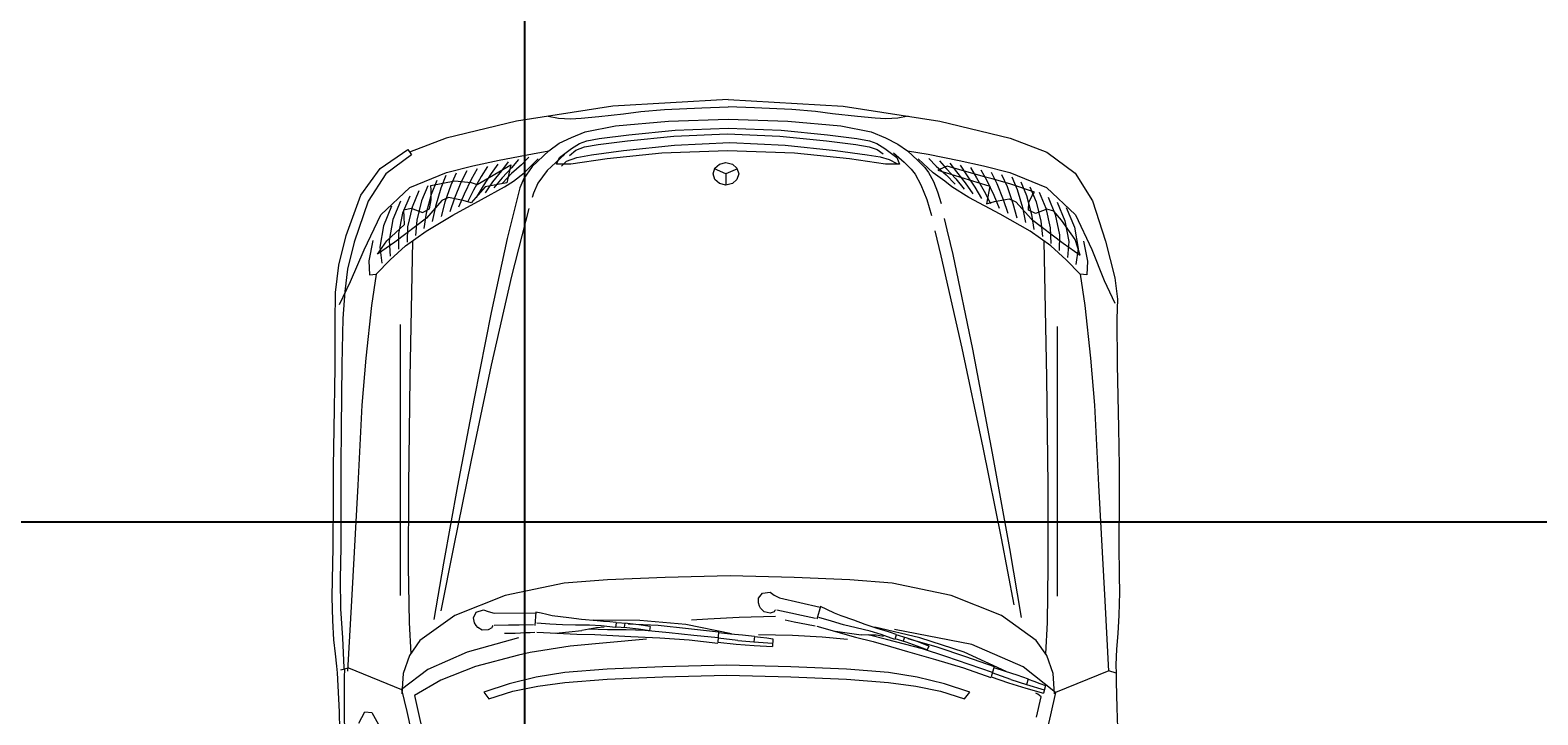
# Model space of a CAD drawing. Units: inches. Extents: x -4347 to -3836, y 955 to 1521.
# Tile 5 of 11: x -4144 to -4072, y 1088 to 1120. Entities that reach past the tile are written whole.
import ezdxf

# ---------------------------------------------------------------- set-up
doc = ezdxf.new("R2010")
doc.units = ezdxf.units.IN
doc.header["$MEASUREMENT"] = 0
doc.layers.add('A-ANNO-DIMS', color=2, linetype='Continuous', lineweight=18)
doc.layers.add('A-SITE-VEHC', color=8, linetype='Continuous', lineweight=13)
doc.styles.get("Standard").update_dxf_attribs({"font": 'arial.ttf'})
doc.dimstyles.get("Standard").update_dxf_attribs({"dimtxt": 0.18, "dimasz": 0.18, "dimexe": 0.18, "dimexo": 0.0625, "dimgap": 0.09, "dimtad": 0, "dimtih": 1, "dimtoh": 1, "dimdec": 0, "dimzin": 0, "dimdsep": 46, "dimlunit": 3, "dimtxsty": 'Standard', "dimcen": 0.09, "dimadec": 0, "dimazin": 0, "dimtfac": 1, "dimtdec": 0, "dimtofl": 0, "dimtmove": 0, "dimatfit": 3, "dimfxl": 1, "dimtolj": 1, "dimtzin": 0, "dimarcsym": 0})

# ---------------------------------------------------------------- blocks, each defined once
blk = doc.blocks.new('*D47')
at = {"layer": 'A-ANNO-DIMS', "color": 0, "lineweight": -2, "transparency": 16777216}
for p, q in [((-4120.58, 1288.726), (-4120.58, 966.959)), ((-3940.58, 1288.726), (-3940.58, 966.959)), ((-4120.4, 967.139), (-4030.97, 967.139)), ((-3940.76, 967.139), (-4030.189, 967.139))]:
    blk.add_line(p, q, dxfattribs=at)
at = {"layer": 'A-ANNO-DIMS', "color": 0, "transparency": 16777216}
for points in [[(-4120.4, 967.169), (-4120.4, 967.109), (-4120.58, 967.139)], [(-3940.76, 967.169), (-3940.76, 967.109), (-3940.58, 967.139)]]:
    blk.add_solid(points, dxfattribs=at)
at = {"layer": 'Defpoints', "color": 0, "transparency": 16777216}
for p in [(-4120.58, 1288.789), (-3940.58, 1288.789), (-3940.58, 967.139)]:
    blk.add_point(p, dxfattribs=at)
at = {"layer": 'A-ANNO-DIMS', "color": 0, "transparency": 16777216, "insert": (-4030.58, 967.139), "char_height": 0.18, "attachment_point": 5}
blk.add_mtext('\\A1;15\'-0"', dxfattribs=at)
blk = doc.blocks.new('*D54')
at = {"layer": 'A-ANNO-DIMS', "color": 0, "lineweight": -2, "transparency": 16777216}
for p, q in [((-3997.757, 1126.789), (-4346.41, 1126.789)), ((-4346.23, 1126.609), (-4346.23, 1111.971)), ((-4346.23, 1096.969), (-4346.23, 1111.607)), ((-3997.757, 1096.789), (-4346.41, 1096.789))]:
    blk.add_line(p, q, dxfattribs=at)
at = {"layer": 'A-ANNO-DIMS', "color": 0, "transparency": 16777216}
for points in [[(-4346.26, 1126.609), (-4346.2, 1126.609), (-4346.23, 1126.789)], [(-4346.26, 1096.969), (-4346.2, 1096.969), (-4346.23, 1096.789)]]:
    blk.add_solid(points, dxfattribs=at)
at = {"layer": 'Defpoints', "color": 0, "transparency": 16777216}
for p in [(-4346.23, 1126.789), (-3997.694, 1126.789), (-3997.694, 1096.789)]:
    blk.add_point(p, dxfattribs=at)
at = {"layer": 'A-ANNO-DIMS', "color": 0, "transparency": 16777216, "insert": (-4346.23, 1111.789), "char_height": 0.18, "attachment_point": 5}
blk.add_mtext('\\A1;2\'-6"', dxfattribs=at)

msp = doc.modelspace()

# ---------------------------------------------------------------- linework, layer by layer
at = {"layer": 'A-SITE-VEHC'}
for p, q in [((-4116.37, 1116.55), (-4120.954, 1115.852)), ((-4110.897, 1116.877), (-4116.37, 1116.55)), ((-4115.864, 1116.196), (-4115.051, 1116.304)), ((-4115.051, 1116.304), (-4113.926, 1116.391)), ((-4113.926, 1116.391), (-4112.141, 1116.479)), ((-4112.141, 1116.479), (-4110.897, 1116.518)), ((-4110.897, 1116.877), (-4105.424, 1116.55)), ((-4109.653, 1116.479), (-4110.897, 1116.518)), ((-4107.868, 1116.391), (-4109.653, 1116.479)), ((-4106.744, 1116.304), (-4107.868, 1116.391)), ((-4105.931, 1116.196), (-4106.744, 1116.304)), ((-4105.424, 1116.55), (-4100.84, 1115.852)), ((-4120.954, 1115.852), (-4124.296, 1115.039)), ((-4119.455, 1116.089), (-4118.967, 1115.989)), ((-4118.967, 1115.989), (-4118.391, 1115.962)), ((-4118.391, 1115.962), (-4117.879, 1115.982)), ((-4117.879, 1115.982), (-4117.043, 1116.065)), ((-4117.7, 1115.337), (-4116.247, 1115.622)), ((-4117.043, 1116.065), (-4115.864, 1116.196)), ((-4116.247, 1115.622), (-4113.735, 1115.851)), ((-4113.735, 1115.851), (-4110.897, 1115.946)), ((-4110.897, 1115.946), (-4108.059, 1115.851)), ((-4108.059, 1115.851), (-4105.548, 1115.622)), ((-4104.752, 1116.065), (-4105.931, 1116.196)), ((-4105.548, 1115.622), (-4104.094, 1115.337)), ((-4103.915, 1115.982), (-4104.752, 1116.065)), ((-4103.403, 1115.962), (-4103.915, 1115.982)), ((-4102.828, 1115.989), (-4103.403, 1115.962)), ((-4102.34, 1116.089), (-4102.828, 1115.989)), ((-4100.84, 1115.852), (-4097.499, 1115.039)), ((-4124.296, 1115.039), (-4126.043, 1114.37)), ((-4118.924, 1114.804), (-4118.348, 1115.074)), ((-4118.348, 1115.074), (-4117.7, 1115.337)), ((-4117.965, 1114.784), (-4117.62, 1114.916)), ((-4117.62, 1114.916), (-4117.02, 1115.015)), ((-4117.075, 1114.739), (-4115.679, 1114.917)), ((-4117.02, 1115.015), (-4115.623, 1115.192)), ((-4115.679, 1114.917), (-4113.471, 1115.134)), ((-4115.623, 1115.192), (-4113.416, 1115.41)), ((-4113.471, 1115.134), (-4110.952, 1115.24)), ((-4113.45, 1114.701), (-4110.815, 1114.827)), ((-4113.416, 1115.41), (-4110.897, 1115.516)), ((-4110.952, 1115.24), (-4108.434, 1115.134)), ((-4110.897, 1115.516), (-4108.379, 1115.41)), ((-4110.815, 1114.827), (-4108.193, 1114.701)), ((-4108.434, 1115.134), (-4106.226, 1114.917)), ((-4108.379, 1115.41), (-4106.171, 1115.192)), ((-4106.226, 1114.917), (-4104.83, 1114.739)), ((-4106.171, 1115.192), (-4104.775, 1115.015)), ((-4104.775, 1115.015), (-4104.175, 1114.916)), ((-4104.175, 1114.916), (-4103.829, 1114.784)), ((-4104.094, 1115.337), (-4103.428, 1115.047)), ((-4103.428, 1115.047), (-4102.833, 1114.748)), ((-4097.499, 1115.039), (-4095.752, 1114.37)), ((-4127.441, 1113.595), (-4126.119, 1114.497)), ((-4125.945, 1114.246), (-4127.162, 1113.348)), ((-4126.119, 1114.497), (-4125.945, 1114.246)), ((-4121.779, 1113.991), (-4120.197, 1114.296)), ((-4120.37, 1114.128), (-4120.713, 1113.766)), ((-4119.419, 1114.442), (-4120.213, 1113.683)), ((-4120.197, 1114.296), (-4119.419, 1114.442)), ((-4118.67, 1114.257), (-4119.501, 1113.498)), ((-4119.419, 1114.442), (-4118.924, 1114.804)), ((-4119.048, 1113.801), (-4118.919, 1114.116)), ((-4118.919, 1114.116), (-4118.345, 1114.549)), ((-4118.572, 1113.943), (-4118.096, 1114.12)), ((-4118.436, 1114.207), (-4118.138, 1114.468)), ((-4118.345, 1114.549), (-4117.965, 1114.784)), ((-4118.138, 1114.468), (-4117.73, 1114.627)), ((-4118.096, 1114.12), (-4117.389, 1114.249)), ((-4117.73, 1114.627), (-4117.075, 1114.739)), ((-4117.389, 1114.249), (-4115.875, 1114.446)), ((-4114.045, 1114.322), (-4116.646, 1114.06)), ((-4115.875, 1114.446), (-4113.45, 1114.701)), ((-4110.933, 1114.442), (-4114.045, 1114.322)), ((-4107.742, 1114.322), (-4110.933, 1114.442)), ((-4108.193, 1114.701), (-4105.792, 1114.446)), ((-4105.137, 1114.06), (-4107.742, 1114.322)), ((-4105.792, 1114.446), (-4104.292, 1114.249)), ((-4104.83, 1114.739), (-4104.195, 1114.631)), ((-4104.292, 1114.249), (-4103.68, 1114.151)), ((-4104.195, 1114.631), (-4103.812, 1114.493)), ((-4103.829, 1114.784), (-4103.45, 1114.549)), ((-4103.812, 1114.493), (-4103.531, 1114.29)), ((-4103.68, 1114.151), (-4103.25, 1114.025)), ((-4103.45, 1114.549), (-4102.876, 1114.116)), ((-4103.038, 1114.344), (-4102.539, 1113.893)), ((-4102.876, 1114.116), (-4102.747, 1113.801)), ((-4102.833, 1114.748), (-4102.376, 1114.442)), ((-4102.376, 1114.442), (-4101.885, 1113.982)), ((-4102.376, 1114.442), (-4101.398, 1114.269)), ((-4101.398, 1114.269), (-4099.916, 1113.977)), ((-4095.752, 1114.37), (-4094.414, 1113.371)), ((-4128.356, 1112.333), (-4127.441, 1113.595)), ((-4126.032, 1112.694), (-4124.287, 1113.409)), ((-4124.287, 1113.409), (-4123.035, 1113.726)), ((-4123.322, 1113.477), (-4123.596, 1112.936)), ((-4122.83, 1113.586), (-4123.116, 1113.074)), ((-4123.035, 1113.726), (-4121.779, 1113.991)), ((-4122.827, 1112.837), (-4121.225, 1113.767)), ((-4122.338, 1113.694), (-4122.635, 1113.212)), ((-4121.846, 1113.803), (-4122.155, 1113.351)), ((-4121.674, 1113.489), (-4122.091, 1112.962)), ((-4121.354, 1113.911), (-4121.674, 1113.489)), ((-4121.193, 1113.627), (-4121.638, 1113.156)), ((-4121.225, 1113.767), (-4121.421, 1112.919)), ((-4120.862, 1114.02), (-4121.193, 1113.627)), ((-4120.713, 1113.766), (-4121.186, 1113.351)), ((-4120.213, 1113.683), (-4120.614, 1113.126)), ((-4120.593, 1113.391), (-4119.92, 1114.048)), ((-4119.501, 1113.498), (-4119.942, 1112.901)), ((-4118.381, 1113.797), (-4119.048, 1113.801)), ((-4118.822, 1113.713), (-4118.572, 1113.943)), ((-4116.646, 1114.06), (-4118.381, 1113.797)), ((-4111.606, 1113.342), (-4111.523, 1113.611)), ((-4111.001, 1113.342), (-4111.543, 1113.573)), ((-4111.523, 1113.611), (-4111.307, 1113.802)), ((-4111.307, 1113.802), (-4111.001, 1113.875)), ((-4111.001, 1113.875), (-4110.696, 1113.802)), ((-4110.46, 1113.573), (-4111.001, 1113.342)), ((-4110.696, 1113.802), (-4110.48, 1113.611)), ((-4110.48, 1113.611), (-4110.397, 1113.342)), ((-4103.414, 1113.797), (-4105.137, 1114.06)), ((-4102.747, 1113.801), (-4103.414, 1113.797)), ((-4103.25, 1114.025), (-4102.886, 1113.835)), ((-4102.539, 1113.893), (-4102.202, 1113.566)), ((-4102.202, 1113.566), (-4102.017, 1113.323)), ((-4101.885, 1113.982), (-4101.553, 1113.649)), ((-4101.154, 1113.394), (-4101.874, 1114.048)), ((-4101.553, 1113.649), (-4101.373, 1113.403)), ((-4101.373, 1113.403), (-4101.145, 1112.973)), ((-4101.353, 1114.073), (-4101.01, 1113.71)), ((-4100.601, 1112.995), (-4101.154, 1113.394)), ((-4101.01, 1113.71), (-4100.537, 1113.296)), ((-4100.497, 1113.712), (-4100.934, 1113.518)), ((-4100.934, 1113.518), (-4098.458, 1112.757)), ((-4100.861, 1113.965), (-4100.529, 1113.572)), ((-4100.529, 1113.572), (-4100.084, 1113.101)), ((-4098.668, 1113.178), (-4100.497, 1113.712)), ((-4100.369, 1113.856), (-4100.049, 1113.434)), ((-4100.049, 1113.434), (-4099.632, 1112.906)), ((-4099.916, 1113.977), (-4098.759, 1113.726)), ((-4099.877, 1113.748), (-4099.568, 1113.295)), ((-4099.385, 1113.639), (-4099.088, 1113.157)), ((-4098.893, 1113.531), (-4098.607, 1113.019)), ((-4098.759, 1113.726), (-4097.507, 1113.409)), ((-4098.401, 1113.422), (-4098.127, 1112.881)), ((-4097.507, 1113.409), (-4095.762, 1112.694)), ((-4127.162, 1113.348), (-4128.009, 1112.035)), ((-4127.403, 1111.398), (-4126.032, 1112.694)), ((-4125.168, 1112.774), (-4125.465, 1112.063)), ((-4125.033, 1112.782), (-4123.893, 1113.011)), ((-4125.018, 1112.562), (-4125.033, 1112.782)), ((-4124.737, 1113.017), (-4125.011, 1112.361)), ((-4124.306, 1113.26), (-4124.557, 1112.659)), ((-4124.077, 1112.797), (-4124.354, 1111.989)), ((-4123.815, 1113.369), (-4124.077, 1112.797)), ((-4123.596, 1112.936), (-4123.901, 1112.183)), ((-4123.893, 1113.011), (-4123.115, 1112.93)), ((-4123.116, 1113.074), (-4123.449, 1112.378)), ((-4123.115, 1112.93), (-4122.827, 1112.837)), ((-4122.441, 1112.726), (-4123.103, 1111.97)), ((-4122.635, 1113.212), (-4122.996, 1112.572)), ((-4122.544, 1112.767), (-4122.87, 1112.218)), ((-4122.626, 1112.121), (-4121.531, 1112.723)), ((-4122.155, 1113.351), (-4122.544, 1112.767)), ((-4122.091, 1112.962), (-4122.452, 1112.445)), ((-4121.421, 1112.919), (-4122.441, 1112.726)), ((-4121.638, 1113.156), (-4122.034, 1112.673)), ((-4121.186, 1113.351), (-4121.616, 1112.9)), ((-4121.531, 1112.723), (-4121.099, 1112.989)), ((-4120.791, 1112.676), (-4121.397, 1110.266)), ((-4121.099, 1112.989), (-4120.593, 1113.391)), ((-4120.614, 1113.126), (-4120.791, 1112.676)), ((-4119.942, 1112.901), (-4120.146, 1112.429)), ((-4111.523, 1113.073), (-4111.606, 1113.342)), ((-4111.307, 1112.882), (-4111.523, 1113.073)), ((-4111.001, 1112.809), (-4111.307, 1112.882)), ((-4111.001, 1113.342), (-4111.001, 1112.809)), ((-4110.696, 1112.882), (-4111.001, 1112.809)), ((-4110.48, 1113.073), (-4110.696, 1112.882)), ((-4110.397, 1113.342), (-4110.48, 1113.073)), ((-4102.017, 1113.323), (-4101.741, 1112.811)), ((-4101.741, 1112.811), (-4101.459, 1112.12)), ((-4101.145, 1112.973), (-4100.95, 1112.481)), ((-4100.263, 1112.723), (-4100.601, 1112.995)), ((-4100.537, 1113.296), (-4100.107, 1112.845)), ((-4099.457, 1112.223), (-4100.263, 1112.723)), ((-4100.084, 1113.101), (-4099.689, 1112.618)), ((-4099.632, 1112.906), (-4099.271, 1112.39)), ((-4099.568, 1113.295), (-4099.179, 1112.712)), ((-4099.179, 1112.712), (-4098.853, 1112.163)), ((-4099.088, 1113.157), (-4098.727, 1112.517)), ((-4098.348, 1113.101), (-4098.668, 1113.178)), ((-4098.458, 1112.757), (-4098.62, 1111.915)), ((-4098.607, 1113.019), (-4098.274, 1112.323)), ((-4097.51, 1112.866), (-4098.348, 1113.101)), ((-4098.127, 1112.881), (-4097.821, 1112.128)), ((-4097.909, 1113.314), (-4097.646, 1112.742)), ((-4097.646, 1112.742), (-4097.369, 1111.933)), ((-4096.338, 1112.466), (-4097.51, 1112.866)), ((-4097.416, 1113.205), (-4097.165, 1112.604)), ((-4096.986, 1112.962), (-4096.712, 1112.306)), ((-4096.555, 1112.719), (-4096.258, 1112.007)), ((-4095.762, 1112.694), (-4094.391, 1111.398)), ((-4094.414, 1113.371), (-4093.591, 1112.065)), ((-4129.051, 1110.416), (-4128.356, 1112.333)), ((-4128.009, 1112.035), (-4128.676, 1110.101)), ((-4126.46, 1112.045), (-4126.826, 1111.168)), ((-4126.03, 1112.288), (-4126.373, 1111.466)), ((-4125.599, 1112.531), (-4125.919, 1111.764)), ((-4125.465, 1112.063), (-4125.688, 1111.147)), ((-4125.011, 1112.361), (-4125.248, 1111.471)), ((-4124.496, 1112.067), (-4125.24, 1111.237)), ((-4125.094, 1111.676), (-4125.017, 1112.098)), ((-4125.017, 1112.098), (-4125.018, 1112.562)), ((-4124.557, 1112.659), (-4124.807, 1111.794)), ((-4124.354, 1111.989), (-4124.542, 1111.308)), ((-4124.184, 1112.214), (-4124.496, 1112.067)), ((-4123.489, 1112.081), (-4124.184, 1112.214)), ((-4123.901, 1112.183), (-4124.124, 1111.535)), ((-4123.973, 1111.37), (-4122.626, 1112.121)), ((-4123.449, 1112.378), (-4123.706, 1111.763)), ((-4123.103, 1111.97), (-4123.489, 1112.081)), ((-4122.996, 1112.572), (-4123.288, 1111.99)), ((-4120.146, 1112.429), (-4120.217, 1112.209)), ((-4101.459, 1112.12), (-4101.232, 1111.354)), ((-4100.95, 1112.481), (-4100.779, 1111.939)), ((-4097.966, 1111.421), (-4099.457, 1112.223)), ((-4098.727, 1112.517), (-4098.435, 1111.935)), ((-4098.62, 1111.915), (-4098.234, 1112.026)), ((-4098.274, 1112.323), (-4098.017, 1111.708)), ((-4098.234, 1112.026), (-4097.539, 1112.158)), ((-4097.821, 1112.128), (-4097.599, 1111.48)), ((-4097.539, 1112.158), (-4097.227, 1112.012)), ((-4097.227, 1112.012), (-4096.483, 1111.182)), ((-4097.165, 1112.604), (-4096.916, 1111.739)), ((-4096.712, 1112.306), (-4096.475, 1111.416)), ((-4096.629, 1111.621), (-4096.614, 1111.975)), ((-4096.614, 1111.975), (-4096.444, 1112.315)), ((-4096.444, 1112.315), (-4096.338, 1112.466)), ((-4096.258, 1112.007), (-4096.035, 1111.092)), ((-4096.124, 1112.476), (-4095.804, 1111.709)), ((-4095.693, 1112.233), (-4095.35, 1111.411)), ((-4095.262, 1111.99), (-4094.897, 1111.113)), ((-4093.591, 1112.065), (-4092.959, 1110.145)), ((-4128.2, 1109.737), (-4127.403, 1111.398)), ((-4126.891, 1111.802), (-4127.28, 1110.87)), ((-4126.373, 1111.466), (-4126.569, 1110.5)), ((-4126.305, 1111.628), (-4125.962, 1111.715)), ((-4126.278, 1110.928), (-4126.305, 1111.628)), ((-4125.919, 1111.764), (-4126.129, 1110.824)), ((-4125.962, 1111.715), (-4125.43, 1111.508)), ((-4125.43, 1111.508), (-4125.094, 1111.676)), ((-4125.248, 1111.471), (-4125.359, 1110.749)), ((-4125.255, 1110.611), (-4123.973, 1111.37)), ((-4124.807, 1111.794), (-4124.96, 1111.08)), ((-4120.372, 1111.698), (-4121.198, 1108.48)), ((-4096.539, 1110.611), (-4097.966, 1111.421)), ((-4097.369, 1111.933), (-4097.181, 1111.253)), ((-4096.916, 1111.739), (-4096.763, 1111.025)), ((-4096.293, 1111.453), (-4096.629, 1111.621)), ((-4096.475, 1111.416), (-4096.364, 1110.694)), ((-4095.761, 1111.66), (-4096.293, 1111.453)), ((-4095.804, 1111.709), (-4095.594, 1110.769)), ((-4095.418, 1111.572), (-4095.761, 1111.66)), ((-4095.051, 1111.132), (-4095.418, 1111.572)), ((-4095.35, 1111.411), (-4095.153, 1110.445)), ((-4094.831, 1111.747), (-4094.443, 1110.814)), ((-4094.391, 1111.398), (-4093.618, 1109.753)), ((-4127.28, 1110.87), (-4127.451, 1109.853)), ((-4127.12, 1110.15), (-4126.278, 1110.928)), ((-4126.826, 1111.168), (-4127.01, 1110.177)), ((-4125.24, 1111.237), (-4126.738, 1110.099)), ((-4126.226, 1109.922), (-4125.255, 1110.611)), ((-4126.129, 1110.824), (-4126.157, 1110.087)), ((-4125.688, 1111.147), (-4125.758, 1110.418)), ((-4101.072, 1110.626), (-4100.979, 1110.232)), ((-4100.625, 1111.216), (-4100.501, 1110.684)), ((-4100.501, 1110.684), (-4100.344, 1110.033)), ((-4095.569, 1109.922), (-4096.539, 1110.611)), ((-4096.483, 1111.182), (-4094.985, 1110.044)), ((-4096.035, 1111.092), (-4095.965, 1110.363)), ((-4095.594, 1110.769), (-4095.566, 1110.032)), ((-4094.406, 1110.224), (-4095.051, 1111.132)), ((-4094.897, 1111.113), (-4094.713, 1110.122)), ((-4094.443, 1110.814), (-4094.272, 1109.798)), ((-4129.391, 1108.996), (-4129.051, 1110.416)), ((-4128.676, 1110.101), (-4128.981, 1108.817)), ((-4127.777, 1110.173), (-4127.971, 1109.21)), ((-4127.556, 1109.526), (-4127.12, 1110.15)), ((-4126.738, 1110.099), (-4127.556, 1109.526)), ((-4127.451, 1109.853), (-4127.354, 1109.094)), ((-4127.01, 1110.177), (-4126.955, 1109.425)), ((-4126.958, 1109.258), (-4126.226, 1109.922)), ((-4126.569, 1110.5), (-4126.556, 1109.756)), ((-4125.9, 1110.145), (-4126.021, 1103.664)), ((-4121.397, 1110.266), (-4122.153, 1106.751)), ((-4100.979, 1110.232), (-4100.888, 1109.836)), ((-4100.888, 1109.836), (-4100.795, 1109.441)), ((-4100.344, 1110.033), (-4100.219, 1109.5)), ((-4095.895, 1110.145), (-4095.774, 1103.664)), ((-4094.837, 1109.258), (-4095.569, 1109.922)), ((-4095.153, 1110.445), (-4095.167, 1109.701)), ((-4094.985, 1110.044), (-4094.167, 1109.471)), ((-4094.713, 1110.122), (-4094.768, 1109.369)), ((-4094.167, 1109.471), (-4094.406, 1110.224)), ((-4094.008, 1110.139), (-4093.822, 1109.189)), ((-4092.959, 1110.145), (-4092.525, 1108.401)), ((-4128.838, 1108.226), (-4128.2, 1109.737)), ((-4127.971, 1109.21), (-4127.941, 1108.539)), ((-4127.618, 1108.57), (-4126.958, 1109.258)), ((-4100.795, 1109.441), (-4099.797, 1105.057)), ((-4100.219, 1109.5), (-4099.288, 1105.007)), ((-4094.176, 1108.57), (-4094.837, 1109.258)), ((-4094.272, 1109.798), (-4094.369, 1109.039)), ((-4093.822, 1109.189), (-4093.856, 1108.535)), ((-4093.618, 1109.753), (-4093.025, 1108.272)), ((-4129.558, 1107.702), (-4129.391, 1108.996)), ((-4128.981, 1108.817), (-4129.121, 1107.746)), ((-4127.941, 1108.539), (-4127.618, 1108.57)), ((-4127.618, 1108.57), (-4127.842, 1107.09)), ((-4121.198, 1108.48), (-4122.152, 1104.256)), ((-4094.176, 1108.57), (-4093.952, 1107.09)), ((-4093.856, 1108.535), (-4094.176, 1108.57)), ((-4092.525, 1108.401), (-4092.402, 1107.389)), ((-4129.575, 1106.28), (-4129.558, 1107.702)), ((-4129.373, 1107.138), (-4128.838, 1108.226)), ((-4129.121, 1107.746), (-4129.207, 1106.463)), ((-4093.025, 1108.272), (-4092.515, 1107.199)), ((-4127.842, 1107.09), (-4128.122, 1104.584)), ((-4093.952, 1107.09), (-4093.672, 1104.584)), ((-4092.402, 1107.389), (-4092.422, 1106.457)), ((-4129.577, 1104.141), (-4129.575, 1106.28)), ((-4129.207, 1106.463), (-4129.263, 1104.276)), ((-4122.153, 1106.751), (-4122.969, 1102.657)), ((-4092.422, 1106.457), (-4092.41, 1104.272)), ((-4126.465, 1093.308), (-4126.465, 1106.181)), ((-4095.239, 1093.269), (-4095.239, 1106.09)), ((-4099.797, 1105.057), (-4098.792, 1100.34)), ((-4099.288, 1105.007), (-4098.345, 1100.07)), ((-4129.619, 1101.221), (-4129.577, 1104.141)), ((-4129.263, 1104.276), (-4129.293, 1101.269)), ((-4128.122, 1104.584), (-4128.298, 1102.34)), ((-4122.152, 1104.256), (-4123.112, 1099.73)), ((-4093.672, 1104.584), (-4093.496, 1102.34)), ((-4092.41, 1104.272), (-4092.35, 1101.267)), ((-4126.021, 1103.664), (-4126.085, 1098.526)), ((-4095.774, 1103.664), (-4095.71, 1098.526)), ((-4122.969, 1102.657), (-4123.755, 1098.509)), ((-4128.298, 1102.34), (-4128.499, 1098.538)), ((-4093.496, 1102.34), (-4093.296, 1098.538)), ((-4129.646, 1099.439), (-4129.619, 1101.221)), ((-4129.293, 1101.269), (-4129.302, 1099.439)), ((-4092.35, 1101.267), (-4092.314, 1099.439)), ((-4098.792, 1100.34), (-4097.919, 1096.027)), ((-4098.345, 1100.07), (-4097.528, 1095.54)), ((-4129.653, 1097.912), (-4129.646, 1099.439)), ((-4129.302, 1099.439), (-4129.301, 1097.918)), ((-4123.112, 1099.73), (-4123.955, 1095.603)), ((-4092.314, 1099.439), (-4092.322, 1097.958)), ((-4128.499, 1098.538), (-4128.802, 1093.049)), ((-4126.085, 1098.526), (-4126.096, 1094.667)), ((-4123.755, 1098.509), (-4124.422, 1094.833)), ((-4095.71, 1098.526), (-4095.699, 1094.667)), ((-4093.296, 1098.538), (-4092.992, 1093.049)), ((-4129.672, 1095.572), (-4129.653, 1097.912)), ((-4129.301, 1097.918), (-4129.305, 1095.591)), ((-4092.322, 1097.958), (-4092.33, 1095.705)), ((-4129.703, 1094.069), (-4129.672, 1095.572)), ((-4129.305, 1095.591), (-4129.327, 1094.094)), ((-4123.955, 1095.603), (-4124.557, 1092.577)), ((-4097.919, 1096.027), (-4097.317, 1092.853)), ((-4097.528, 1095.54), (-4096.971, 1092.264)), ((-4092.33, 1095.705), (-4092.314, 1094.248)), ((-4124.422, 1094.833), (-4124.879, 1092.154)), ((-4129.716, 1093.228), (-4129.703, 1094.069)), ((-4129.327, 1094.094), (-4129.325, 1092.672)), ((-4126.096, 1094.667), (-4126.057, 1092.021)), ((-4116.633, 1094.048), (-4118.685, 1093.89)), ((-4113.893, 1094.152), (-4116.633, 1094.048)), ((-4110.799, 1094.232), (-4113.893, 1094.152)), ((-4107.756, 1094.152), (-4110.799, 1094.232)), ((-4105.111, 1094.048), (-4107.756, 1094.152)), ((-4103.11, 1093.89), (-4105.111, 1094.048)), ((-4095.699, 1094.667), (-4095.738, 1092.021)), ((-4092.314, 1094.248), (-4092.301, 1093.437)), ((-4118.685, 1093.89), (-4121.501, 1093.303)), ((-4109.453, 1093.178), (-4109.269, 1093.418)), ((-4109.269, 1093.418), (-4108.906, 1093.457)), ((-4108.906, 1093.457), (-4108.703, 1093.315)), ((-4100.294, 1093.303), (-4103.11, 1093.89)), ((-4092.301, 1093.437), (-4092.328, 1092.373)), ((-4129.689, 1092.112), (-4129.716, 1093.228)), ((-4129.325, 1092.672), (-4129.22, 1091.286)), ((-4128.802, 1093.049), (-4128.979, 1089.7)), ((-4121.501, 1093.303), (-4123.883, 1092.351)), ((-4122.869, 1092.508), (-4122.525, 1092.628)), ((-4122.525, 1092.628), (-4122.295, 1092.535)), ((-4109.459, 1092.947), (-4109.453, 1093.178)), ((-4109.413, 1092.798), (-4109.459, 1092.947)), ((-4109.356, 1092.7), (-4109.413, 1092.798)), ((-4109.186, 1092.528), (-4109.356, 1092.7)), ((-4108.703, 1093.315), (-4108.455, 1093.184)), ((-4108.641, 1092.619), (-4108.677, 1092.592)), ((-4108.455, 1093.184), (-4106.525, 1092.749)), ((-4106.515, 1092.779), (-4106.691, 1092.178)), ((-4106.211, 1092.64), (-4106.515, 1092.779)), ((-4105.841, 1092.457), (-4106.211, 1092.64)), ((-4097.911, 1092.351), (-4100.294, 1093.303)), ((-4092.992, 1093.049), (-4092.816, 1089.7)), ((-4129.63, 1091.199), (-4129.689, 1092.112)), ((-4126.057, 1092.021), (-4125.971, 1090.524)), ((-4123.883, 1092.351), (-4125.542, 1091.168)), ((-4122.995, 1092.233), (-4122.869, 1092.508)), ((-4122.948, 1092.006), (-4122.995, 1092.233)), ((-4122.871, 1091.871), (-4122.948, 1092.006)), ((-4122.295, 1092.535), (-4122.024, 1092.463)), ((-4122.024, 1092.463), (-4120.045, 1092.473)), ((-4120.141, 1091.903), (-4120.826, 1091.893)), ((-4120.042, 1092.505), (-4120.078, 1091.879)), ((-4119.787, 1092.455), (-4120.042, 1092.505)), ((-4119.372, 1091.944), (-4119.989, 1091.985)), ((-4119.52, 1092.391), (-4119.787, 1092.455)), ((-4119.264, 1092.343), (-4119.52, 1092.391)), ((-4118.777, 1091.904), (-4119.372, 1091.944)), ((-4118.467, 1092.236), (-4119.264, 1092.343)), ((-4118.158, 1091.898), (-4118.777, 1091.904)), ((-4117.866, 1092.156), (-4118.467, 1092.236)), ((-4117.481, 1091.899), (-4118.158, 1091.898)), ((-4117.122, 1092.093), (-4117.866, 1092.156)), ((-4116.932, 1091.854), (-4117.481, 1091.899)), ((-4115.094, 1092.118), (-4117.298, 1092.135)), ((-4116.825, 1092.07), (-4117.122, 1092.093)), ((-4116.522, 1092.043), (-4116.825, 1092.07)), ((-4116.226, 1092.02), (-4116.522, 1092.043)), ((-4116.222, 1092.001), (-4116.243, 1091.779)), ((-4115.688, 1091.974), (-4116.234, 1092.008)), ((-4115.813, 1091.981), (-4115.832, 1091.791)), ((-4115.14, 1091.906), (-4115.688, 1091.974)), ((-4115.652, 1091.956), (-4114.219, 1091.89)), ((-4114.598, 1091.827), (-4115.14, 1091.906)), ((-4112.901, 1091.924), (-4115.094, 1092.118)), ((-4110.743, 1091.486), (-4112.901, 1091.924)), ((-4111.857, 1092.176), (-4112.646, 1092.136)), ((-4110.369, 1092.259), (-4111.857, 1092.176)), ((-4108.643, 1092.311), (-4110.369, 1092.259)), ((-4108.903, 1092.467), (-4109.186, 1092.528)), ((-4108.707, 1092.531), (-4108.903, 1092.467)), ((-4108.677, 1092.592), (-4108.707, 1092.531)), ((-4107.916, 1092.466), (-4108.586, 1092.605)), ((-4108.189, 1092.144), (-4107.764, 1092.046)), ((-4107.416, 1092.359), (-4107.916, 1092.466)), ((-4107.764, 1092.046), (-4107.182, 1091.935)), ((-4106.747, 1092.215), (-4107.416, 1092.359)), ((-4107.182, 1091.935), (-4106.767, 1091.862)), ((-4105.988, 1092.082), (-4106.581, 1092.26)), ((-4105.418, 1091.909), (-4105.988, 1092.082)), ((-4105.533, 1092.329), (-4105.841, 1092.457)), ((-4104.919, 1092.122), (-4105.533, 1092.329)), ((-4104.816, 1091.764), (-4105.418, 1091.909)), ((-4104.389, 1091.919), (-4104.919, 1092.122)), ((-4103.763, 1091.721), (-4104.389, 1091.919)), ((-4096.253, 1091.168), (-4097.911, 1092.351)), ((-4095.738, 1092.021), (-4095.823, 1090.524)), ((-4092.328, 1092.373), (-4092.386, 1091.491)), ((-4129.556, 1090.526), (-4129.63, 1091.199)), ((-4129.22, 1091.286), (-4129.158, 1089.867)), ((-4120.863, 1091.29), (-4123.306, 1090.616)), ((-4122.793, 1091.789), (-4122.871, 1091.871)), ((-4122.588, 1091.66), (-4122.793, 1091.789)), ((-4122.299, 1091.664), (-4122.588, 1091.66)), ((-4122.122, 1091.77), (-4122.299, 1091.664)), ((-4122.107, 1091.836), (-4122.122, 1091.77)), ((-4122.078, 1091.87), (-4122.107, 1091.836)), ((-4121.337, 1091.885), (-4122.021, 1091.869)), ((-4121.53, 1091.51), (-4121.275, 1091.505)), ((-4120.826, 1091.893), (-4121.337, 1091.885)), ((-4121.275, 1091.505), (-4121.015, 1091.518)), ((-4121.015, 1091.518), (-4120.759, 1091.533)), ((-4120.759, 1091.533), (-4120.533, 1091.539)), ((-4120.533, 1091.539), (-4120.307, 1091.545)), ((-4120.307, 1091.545), (-4120.082, 1091.555)), ((-4119.991, 1091.565), (-4118.083, 1091.457)), ((-4119.08, 1091.517), (-4117.845, 1091.636)), ((-4114.782, 1091.222), (-4118.398, 1090.891)), ((-4118.083, 1091.457), (-4117.231, 1091.449)), ((-4117.496, 1091.701), (-4117.845, 1091.636)), ((-4116.634, 1091.677), (-4117.518, 1091.701)), ((-4117.148, 1091.772), (-4117.496, 1091.701)), ((-4117.231, 1091.449), (-4116.375, 1091.406)), ((-4116.795, 1091.796), (-4117.148, 1091.772)), ((-4116.243, 1091.779), (-4116.932, 1091.854)), ((-4115.749, 1091.665), (-4116.634, 1091.677)), ((-4116.375, 1091.406), (-4115.524, 1091.355)), ((-4116.252, 1091.818), (-4115.708, 1091.782)), ((-4114.864, 1091.631), (-4115.749, 1091.665)), ((-4115.708, 1091.782), (-4115.16, 1091.72)), ((-4115.524, 1091.355), (-4114.149, 1091.284)), ((-4115.16, 1091.72), (-4114.619, 1091.646)), ((-4113.698, 1091.532), (-4114.864, 1091.631)), ((-4114.598, 1091.827), (-4114.629, 1091.644)), ((-4114.219, 1091.89), (-4112.784, 1091.738)), ((-4114.149, 1091.284), (-4112.752, 1091.191)), ((-4112.534, 1091.407), (-4113.698, 1091.532)), ((-4112.784, 1091.738), (-4111.355, 1091.583)), ((-4112.752, 1091.191), (-4111.384, 1091.038)), ((-4111.37, 1091.289), (-4112.534, 1091.407)), ((-4111.355, 1091.583), (-4111.384, 1091.079)), ((-4110.441, 1091.163), (-4111.378, 1091.277)), ((-4111.356, 1091.541), (-4110.788, 1091.483)), ((-4110.788, 1091.483), (-4110.219, 1091.433)), ((-4110.219, 1091.433), (-4109.651, 1091.376)), ((-4109.647, 1091.356), (-4109.671, 1091.102)), ((-4109.647, 1091.356), (-4109.356, 1091.325)), ((-4107.841, 1091.405), (-4109.452, 1091.434)), ((-4109.356, 1091.325), (-4109.064, 1091.289)), ((-4109.064, 1091.289), (-4108.774, 1091.247)), ((-4108.774, 1091.247), (-4108.79, 1090.871)), ((-4106.424, 1091.322), (-4107.841, 1091.405)), ((-4106.677, 1091.852), (-4104.842, 1091.317)), ((-4105.223, 1091.207), (-4106.424, 1091.322)), ((-4105.799, 1091.6), (-4104.569, 1091.438)), ((-4104.842, 1091.317), (-4104.013, 1091.118)), ((-4104.156, 1091.613), (-4104.816, 1091.764)), ((-4104.215, 1091.423), (-4104.569, 1091.438)), ((-4103.38, 1091.205), (-4104.237, 1091.428)), ((-4103.86, 1091.413), (-4104.215, 1091.423)), ((-4103.631, 1091.445), (-4104.156, 1091.613)), ((-4101.781, 1091.289), (-4103.924, 1091.801)), ((-4103.511, 1091.358), (-4103.86, 1091.413)), ((-4103.477, 1091.635), (-4103.763, 1091.721)), ((-4102.976, 1091.217), (-4103.631, 1091.445)), ((-4103.189, 1091.539), (-4103.477, 1091.635)), ((-4102.52, 1090.995), (-4103.38, 1091.205)), ((-4102.906, 1091.449), (-4103.189, 1091.539)), ((-4099.319, 1090.97), (-4102.999, 1091.684)), ((-4102.906, 1091.428), (-4102.976, 1091.217)), ((-4102.976, 1091.257), (-4102.454, 1091.099)), ((-4102.392, 1091.282), (-4102.916, 1091.438)), ((-4102.513, 1091.317), (-4102.573, 1091.136)), ((-4101.873, 1091.093), (-4102.392, 1091.282)), ((-4102.361, 1091.257), (-4100.98, 1090.87)), ((-4099.688, 1090.607), (-4101.781, 1091.289)), ((-4092.386, 1091.491), (-4092.444, 1090.744)), ((-4129.493, 1089.939), (-4129.556, 1090.526)), ((-4125.542, 1091.168), (-4126.041, 1090.455)), ((-4123.306, 1090.616), (-4125.161, 1089.788)), ((-4120.306, 1090.592), (-4120.863, 1090.463)), ((-4118.398, 1090.891), (-4120.306, 1090.592)), ((-4111.384, 1091.079), (-4110.52, 1090.986)), ((-4110.52, 1090.986), (-4109.658, 1090.918)), ((-4110.441, 1091.163), (-4109.671, 1091.102)), ((-4109.671, 1091.102), (-4108.787, 1091.037)), ((-4109.658, 1090.918), (-4108.79, 1090.871)), ((-4104.013, 1091.118), (-4103.19, 1090.883)), ((-4103.19, 1090.883), (-4102.371, 1090.642)), ((-4101.666, 1090.763), (-4102.52, 1090.995)), ((-4102.454, 1091.099), (-4101.935, 1090.916)), ((-4102.371, 1090.642), (-4101.047, 1090.264)), ((-4101.935, 1090.916), (-4101.424, 1090.723)), ((-4101.363, 1090.894), (-4101.873, 1091.093)), ((-4100.552, 1090.404), (-4101.666, 1090.763)), ((-4101.363, 1090.894), (-4101.434, 1090.723)), ((-4100.98, 1090.87), (-4099.615, 1090.399)), ((-4097.683, 1089.694), (-4099.688, 1090.607)), ((-4096.879, 1089.914), (-4099.319, 1090.97)), ((-4095.753, 1090.455), (-4096.253, 1091.168)), ((-4092.444, 1090.744), (-4092.471, 1090.005)), ((-4129.463, 1089.625), (-4129.493, 1089.939)), ((-4129.3, 1089.765), (-4128.944, 1089.872)), ((-4129.158, 1089.867), (-4129.146, 1089.838)), ((-4129.146, 1089.838), (-4129.138, 1089.805)), ((-4129.134, 1089.769), (-4129.143, 1089.453)), ((-4129.138, 1089.805), (-4129.134, 1089.769)), ((-4128.944, 1089.872), (-4126.417, 1088.84)), ((-4125.161, 1089.788), (-4126.417, 1088.84)), ((-4126.041, 1090.455), (-4126.334, 1089.593)), ((-4122.899, 1089.926), (-4124.545, 1089.282)), ((-4120.863, 1090.463), (-4122.899, 1089.926)), ((-4116.653, 1089.802), (-4118.654, 1089.644)), ((-4114.008, 1089.906), (-4116.653, 1089.802)), ((-4110.965, 1089.986), (-4114.008, 1089.906)), ((-4107.921, 1089.906), (-4110.965, 1089.986)), ((-4105.276, 1089.802), (-4107.921, 1089.906)), ((-4103.275, 1089.644), (-4105.276, 1089.802)), ((-4101.047, 1090.264), (-4099.708, 1089.859)), ((-4099.446, 1090.021), (-4100.552, 1090.404)), ((-4099.708, 1089.859), (-4098.409, 1089.402)), ((-4099.615, 1090.399), (-4098.258, 1089.926)), ((-4098.339, 1089.644), (-4099.446, 1090.021)), ((-4098.258, 1089.926), (-4098.399, 1089.442)), ((-4098.268, 1089.886), (-4097.728, 1089.702)), ((-4095.342, 1088.688), (-4096.879, 1089.914)), ((-4095.46, 1089.593), (-4095.753, 1090.455)), ((-4092.471, 1090.005), (-4092.458, 1089.593)), ((-4129.432, 1089.01), (-4129.463, 1089.625)), ((-4129.143, 1089.453), (-4129.151, 1088.327)), ((-4126.334, 1089.593), (-4126.401, 1088.626)), ((-4124.545, 1089.282), (-4125.796, 1088.55)), ((-4121.31, 1089.105), (-4122.515, 1088.704)), ((-4120.013, 1089.422), (-4121.31, 1089.105)), ((-4118.654, 1089.644), (-4120.013, 1089.422)), ((-4119.949, 1088.993), (-4118.654, 1089.175)), ((-4118.654, 1089.175), (-4116.653, 1089.333)), ((-4116.653, 1089.333), (-4114.008, 1089.438)), ((-4114.008, 1089.438), (-4110.965, 1089.517)), ((-4110.965, 1089.517), (-4107.921, 1089.438)), ((-4107.921, 1089.438), (-4105.276, 1089.333)), ((-4105.276, 1089.333), (-4103.275, 1089.175)), ((-4101.916, 1089.422), (-4103.275, 1089.644)), ((-4103.275, 1089.175), (-4101.98, 1088.993)), ((-4100.619, 1089.105), (-4101.916, 1089.422)), ((-4099.414, 1088.704), (-4100.619, 1089.105)), ((-4098.399, 1089.442), (-4097.578, 1089.157)), ((-4097.461, 1089.311), (-4098.349, 1089.634)), ((-4097.728, 1089.702), (-4097.185, 1089.525)), ((-4097.578, 1089.157), (-4096.754, 1088.897)), ((-4097.461, 1089.311), (-4096.725, 1089.079)), ((-4097.185, 1089.525), (-4096.645, 1089.341)), ((-4096.645, 1089.321), (-4096.725, 1089.079)), ((-4096.725, 1089.079), (-4095.879, 1088.817)), ((-4096.645, 1089.321), (-4096.368, 1089.226)), ((-4096.368, 1089.226), (-4096.091, 1089.124)), ((-4096.091, 1089.124), (-4095.818, 1089.019)), ((-4095.394, 1088.626), (-4095.46, 1089.593)), ((-4092.815, 1089.72), (-4095.342, 1088.688)), ((-4092.459, 1089.613), (-4092.815, 1089.72)), ((-4092.458, 1089.593), (-4092.452, 1089.204)), ((-4092.452, 1089.204), (-4092.424, 1087.964)), ((-4129.374, 1087.772), (-4129.432, 1089.01)), ((-4129.151, 1088.327), (-4129.134, 1086.126)), ((-4126.417, 1088.84), (-4126.173, 1087.783)), ((-4125.796, 1088.55), (-4123.555, 1078.317)), ((-4122.515, 1088.704), (-4122.269, 1088.387)), ((-4122.269, 1088.387), (-4121.127, 1088.748)), ((-4121.127, 1088.748), (-4119.949, 1088.993)), ((-4101.98, 1088.993), (-4100.802, 1088.748)), ((-4100.802, 1088.748), (-4099.66, 1088.387)), ((-4099.66, 1088.387), (-4099.414, 1088.704)), ((-4096.754, 1088.897), (-4095.919, 1088.656)), ((-4096.186, 1088.611), (-4096.272, 1088.666)), ((-4096.245, 1087.523), (-4096.02, 1088.485)), ((-4096.102, 1088.55), (-4096.186, 1088.611)), ((-4096.02, 1088.485), (-4096.102, 1088.55)), ((-4095.818, 1089.019), (-4095.919, 1088.656)), ((-4095.342, 1088.688), (-4095.586, 1087.631)), ((-4129.327, 1085.96), (-4129.374, 1087.772)), ((-4128.446, 1087.238), (-4128.158, 1087.781)), ((-4128.158, 1087.781), (-4127.831, 1087.739)), ((-4127.831, 1087.739), (-4127.52, 1087.167)), ((-4126.173, 1087.783), (-4125.652, 1085.508)), ((-4095.586, 1087.631), (-4096.106, 1085.355)), ((-4092.424, 1087.964), (-4092.357, 1085.761))]:
    msp.add_line(p, q, dxfattribs=at)

# ---------------------------------------------------------------- dimensions: what is measured, and where the dimension line sits
at = {"layer": 'A-ANNO-DIMS'}
dim = msp.add_linear_dim(base=(-3940.58, 967.139), p1=(-4120.58, 1288.789), p2=(-3940.58, 1288.789), dimstyle='Standard', override={"dimdec": 1, "dimlfac": 1, "dimrnd": 0, "dimzin": 1, "dimdsep": 46, "dimlunit": 4, "dimfrac": 2}, dxfattribs=at)
dim.commit()
dim.dimension.update_dxf_attribs({"geometry": '*D47', "text_midpoint": (-4030.58, 967.139)})
dim = msp.add_linear_dim(base=(-4346.23, 1126.789), p1=(-3997.694, 1096.789), p2=(-3997.694, 1126.789), angle=90, dimstyle='Standard', override={"dimdec": 1, "dimlfac": 1, "dimrnd": 0, "dimzin": 1, "dimdsep": 46, "dimlunit": 4, "dimfrac": 2}, dxfattribs=at)
dim.commit()
dim.dimension.update_dxf_attribs({"geometry": '*D54', "text_midpoint": (-4346.23, 1111.789)})

doc.saveas('drawing.dxf')
